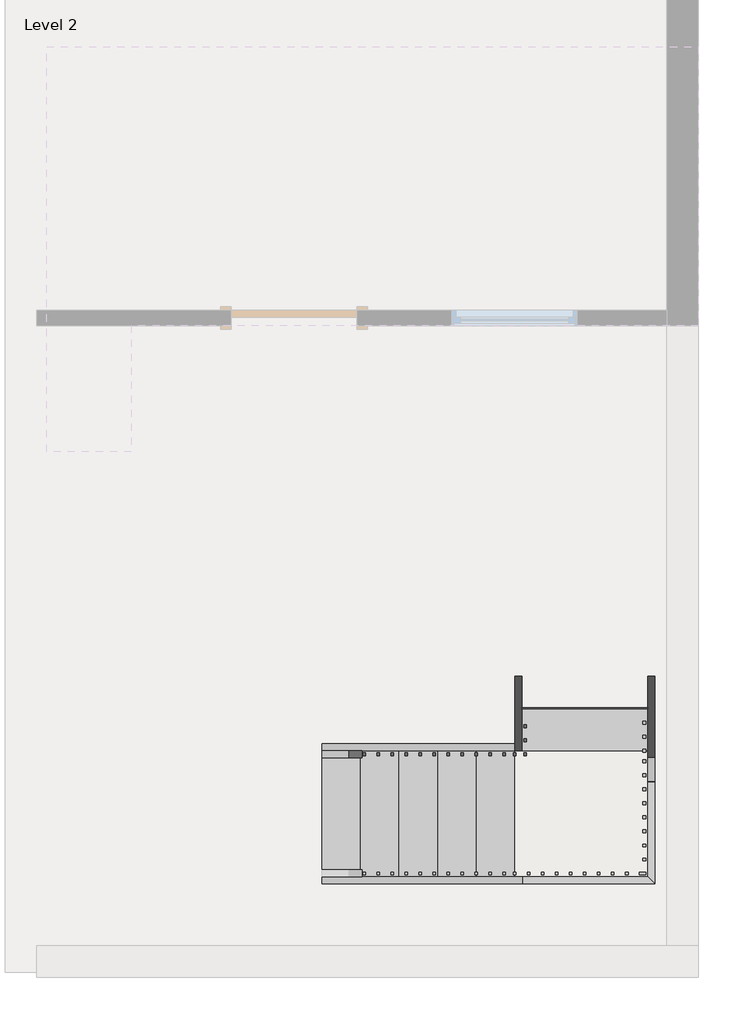
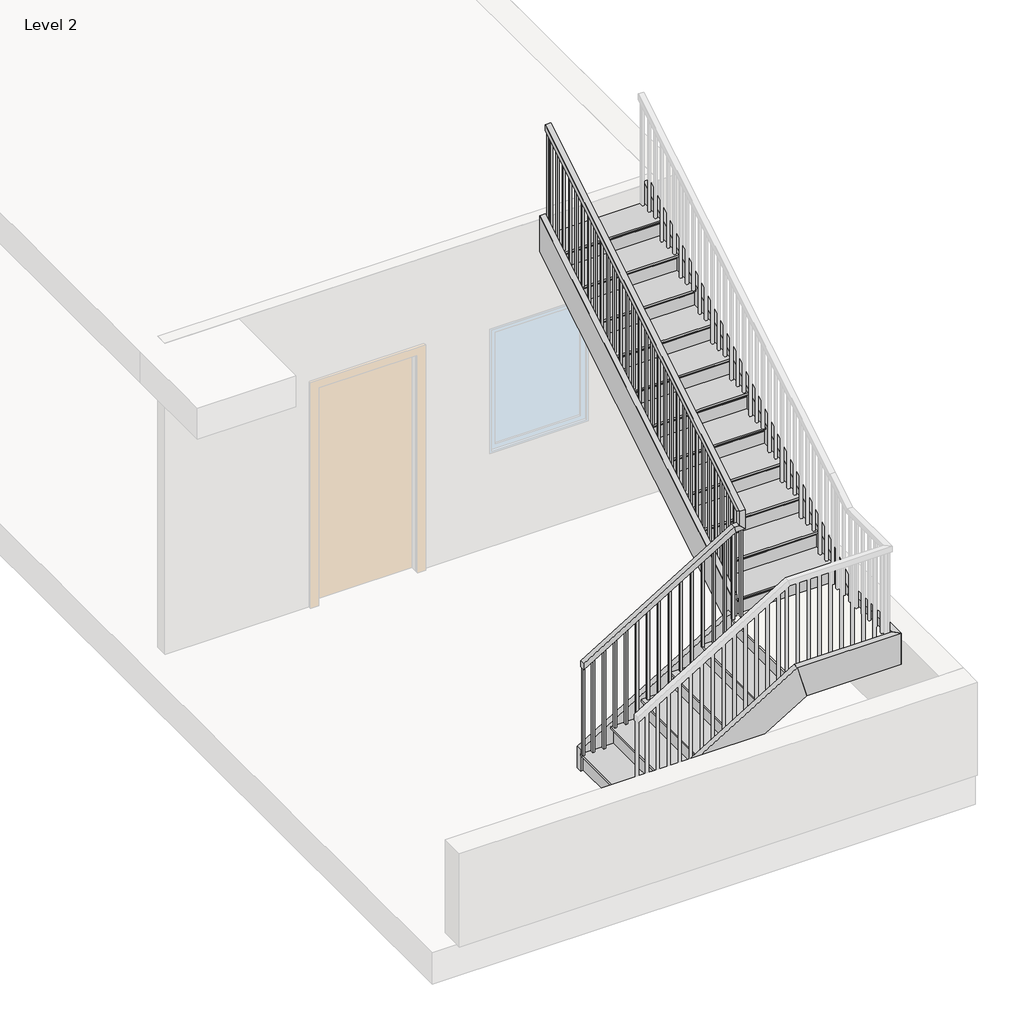
# One storey, part 2 of 2: 6 members, 2 stair flights, 1 railing, 1 slab.
"""IFC4 building model written with IfcOpenShell, lengths in millimetres."""

from ifc_helpers import new_model, si_unit, frame, origin, place, context, project, spatial, polyline, outline, extrude, faceted_brep, transform, mapped, element, save
from components import non_monolithic_landing_5acc3baf, stair_flight_09e20c57, stair_flight_b0062ef7

model = new_model("IFC4")

# Units and contexts
model_context = context("Model", 3, world=origin())
ifc_project = project(units=[si_unit("LENGTHUNIT", "METRE", prefix="MILLI")], contexts=[model_context])

# Site, building, storey
site = spatial("IfcSite", under=ifc_project)
building = spatial("IfcBuilding", under=site)
storey = spatial("IfcBuildingStorey", under=building, Name="Level 2", Elevation=3048.0)

# Members
placement = place(None, origin())
element("IfcMember", 1, ObjectType="Stringer - 2\" Width", at=placement, inside=storey, context=model_context, shape_type="SweptSolid", body=[
    extrude(outline(polyline([(3260.114512, -3351.0563134), (3048.0, -3351.0563134), (3048.0, -3112.9708017), (3750.3724171, -1954.0563134), (4106.7811786, -1954.0563134), (3260.114512, -3351.0563134)])), frame((0.0, -11795.059218, 0.0), z_axis=(0.0, 1.0, 0.0), x_axis=(0.0, 0.0, 1.0)), (0.0, 0.0, 1.0), 50.8),
])
element("IfcMember", 2, ObjectType="Stringer - 2\" Width", at=placement, inside=storey, context=model_context, shape_type="SweptSolid", body=[
    extrude(outline(polyline([(3260.114512, -3351.0563134), (3048.0, -3351.0563134), (3048.0, -3112.9708017), (3835.4, -1813.7608017), (4140.2, -1898.9152582), (3260.114512, -3351.0563134)])), frame((0.0, -12760.259218, 0.0), z_axis=(0.0, 1.0, 0.0), x_axis=(0.0, 0.0, 1.0)), (0.0, 0.0, 1.0), 50.8),
])
element("IfcMember", 3, ObjectType="Stringer - 2\" Width", at=placement, inside=storey, context=model_context, shape_type="SweptSolid", body=[
    extrude(outline(polyline([(-11795.059218, 3919.7057504), (-11795.059218, 4276.114512), (-8721.659218, 6138.7811786), (-8721.659218, 5782.3724171), (-11795.059218, 3919.7057504)])), frame((-1954.0563134, 0.0, 0.0), z_axis=(1.0, 0.0, 0.0), x_axis=(0.0, 1.0, 0.0)), (0.0, 0.0, 1.0), 50.8),
])
element("IfcMember", 4, ObjectType="Stringer - 2\" Width", at=placement, inside=storey, context=model_context, shape_type="SweptSolid", body=[
    extrude(outline(polyline([(-11934.1637062, 3835.4), (-12019.3181627, 4140.2), (-8721.659218, 6138.7811786), (-8721.659218, 5782.3724171), (-11934.1637062, 3835.4)])), frame((-988.8563134, 0.0, 0.0), z_axis=(1.0, 0.0, 0.0), x_axis=(0.0, 1.0, 0.0)), (0.0, 0.0, 1.0), 50.8),
])
element("IfcMember", 5, ObjectType="Stringer - 2\" Width", at=placement, inside=storey, context=model_context, shape_type="Brep", body=[
    faceted_brep([(-1898.9152582, -12709.459218, 4140.2), (-1898.9152582, -12760.259218, 4140.2), (-938.0563134, -12760.259218, 4140.2), (-988.8563134, -12709.459218, 4140.2), (-1813.7608017, -12709.459218, 3835.4), (-988.8563134, -12709.459218, 3835.4), (-1813.7608017, -12760.259218, 3835.4), (-938.0563134, -12760.259218, 3835.4)], [[[0, 1, 2, 3]], [[4, 0, 3, 5]], [[6, 4, 5, 7]], [[1, 6, 7, 2]], [[1, 0, 4, 6]], [[2, 7, 5, 3]]]),
])
element("IfcMember", 6, ObjectType="Stringer - 2\" Width", at=placement, inside=storey, context=model_context, shape_type="Brep", body=[
    faceted_brep([(-988.8563134, -12709.459218, 4140.2), (-938.0563134, -12760.259218, 4140.2), (-938.0563134, -12019.3181627, 4140.2), (-988.8563134, -12019.3181627, 4140.2), (-988.8563134, -12709.459218, 3835.4), (-988.8563134, -11934.1637062, 3835.4), (-938.0563134, -12760.259218, 3835.4), (-938.0563134, -11934.1637062, 3835.4)], [[[0, 1, 2, 3]], [[4, 0, 3, 5]], [[6, 4, 5, 7]], [[1, 6, 7, 2]], [[1, 0, 4, 6]], [[2, 7, 5, 3]]]),
])

# Railing
element("IfcRailing", 7, ObjectType="Handrail - Rectangular", at=placement, inside=storey, context=model_context, shape_type="SolidModel", body=[
    faceted_brep([(-3351.0563134, -11795.059218, 4131.7333333), (-3351.0563134, -11795.059218, 4072.3318731), (-3351.0563134, -11845.859218, 4072.3318731), (-3351.0563134, -11845.859218, 4131.7333333), (-1954.0563134, -11795.059218, 4978.4), (-1939.863904, -11795.059218, 4927.6), (-1939.863904, -11845.859218, 4927.6), (-1954.0563134, -11845.859218, 4978.4), (-1903.2563134, -11795.059218, 4978.4), (-1903.2563134, -11845.859218, 4978.4), (-1852.4563134, -11845.859218, 4927.6), (-1852.4563134, -11795.059218, 4927.6)], [[[0, 1, 2, 3]], [[1, 0, 4, 5]], [[2, 1, 5, 6]], [[3, 2, 6, 7]], [[0, 3, 7, 4]], [[8, 9, 10, 11]], [[5, 4, 8, 11]], [[6, 5, 11, 10]], [[7, 6, 10, 9]], [[4, 7, 9, 8]]]),
    faceted_brep([(-1903.2563134, -11795.059218, 4978.4), (-1852.4563134, -11795.059218, 4927.6), (-1852.4563134, -11845.859218, 4927.6), (-1903.2563134, -11845.859218, 4978.4), (-1903.2563134, -11795.059218, 5088.3318731), (-1903.2563134, -11845.859218, 5116.9454545), (-1852.4563134, -11845.859218, 5116.9454545), (-1852.4563134, -11795.059218, 5088.3318731)], [[[0, 1, 2, 3]], [[4, 5, 6, 7]], [[1, 0, 4, 7]], [[2, 1, 7, 6]], [[3, 2, 6, 5]], [[0, 3, 5, 4]]]),
    faceted_brep([(-1903.2563134, -11845.859218, 5116.9454545), (-1903.2563134, -11795.059218, 5088.3318731), (-1852.4563134, -11795.059218, 5088.3318731), (-1852.4563134, -11845.859218, 5116.9454545), (-1903.2563134, -8721.659218, 7010.4), (-1852.4563134, -8721.659218, 7010.4), (-1852.4563134, -8721.659218, 6950.9985397), (-1903.2563134, -8721.659218, 6950.9985397)], [[[0, 1, 2, 3]], [[4, 5, 6, 7]], [[1, 0, 4, 7]], [[2, 1, 7, 6]], [[3, 2, 6, 5]], [[0, 3, 5, 4]]]),
    extrude(outline(polyline([(-8762.934218, 6925.9833882), (-8762.934218, 5926.6666667), (-8781.984218, 5926.6666667), (-8781.984218, 6914.4379337), (-8762.934218, 6925.9833882)])), frame((-1887.3813134, 0.0, 0.0), z_axis=(1.0, 0.0, 0.0), x_axis=(0.0, 1.0, 0.0)), (0.0, 0.0, 1.0), 19.05),
    extrude(outline(polyline([(-8864.534218, 6864.4076307), (-8864.534218, 5926.6666667), (-8883.584218, 5926.6666667), (-8883.584218, 6852.8621761), (-8864.534218, 6864.4076307)])), frame((-1887.3813134, 0.0, 0.0), z_axis=(1.0, 0.0, 0.0), x_axis=(0.0, 1.0, 0.0)), (0.0, 0.0, 1.0), 19.05),
    extrude(outline(polyline([(-8966.134218, 6802.8318731), (-8966.134218, 5926.6666667), (-8985.184218, 5926.6666667), (-8985.184218, 6791.2864185), (-8966.134218, 6802.8318731)])), frame((-1887.3813134, 0.0, 0.0), z_axis=(1.0, 0.0, 0.0), x_axis=(0.0, 1.0, 0.0)), (0.0, 0.0, 1.0), 19.05),
    extrude(outline(polyline([(-9067.734218, 6741.2561155), (-9067.734218, 5757.3333333), (-9086.784218, 5757.3333333), (-9086.784218, 6729.710661), (-9067.734218, 6741.2561155)])), frame((-1887.3813134, 0.0, 0.0), z_axis=(1.0, 0.0, 0.0), x_axis=(0.0, 1.0, 0.0)), (0.0, 0.0, 1.0), 19.05),
    extrude(outline(polyline([(-9169.334218, 6679.6803579), (-9169.334218, 5757.3333333), (-9188.384218, 5757.3333333), (-9188.384218, 6668.1349034), (-9169.334218, 6679.6803579)])), frame((-1887.3813134, 0.0, 0.0), z_axis=(1.0, 0.0, 0.0), x_axis=(0.0, 1.0, 0.0)), (0.0, 0.0, 1.0), 19.05),
    extrude(outline(polyline([(-9270.934218, 6618.1046004), (-9270.934218, 5757.3333333), (-9289.984218, 5757.3333333), (-9289.984218, 6606.5591458), (-9270.934218, 6618.1046004)])), frame((-1887.3813134, 0.0, 0.0), z_axis=(1.0, 0.0, 0.0), x_axis=(0.0, 1.0, 0.0)), (0.0, 0.0, 1.0), 19.05),
    extrude(outline(polyline([(-9372.534218, 6556.5288428), (-9372.534218, 5588.0), (-9391.584218, 5588.0), (-9391.584218, 6544.9833882), (-9372.534218, 6556.5288428)])), frame((-1887.3813134, 0.0, 0.0), z_axis=(1.0, 0.0, 0.0), x_axis=(0.0, 1.0, 0.0)), (0.0, 0.0, 1.0), 19.05),
    extrude(outline(polyline([(-9474.134218, 6494.9530852), (-9474.134218, 5588.0), (-9493.184218, 5588.0), (-9493.184218, 6483.4076307), (-9474.134218, 6494.9530852)])), frame((-1887.3813134, 0.0, 0.0), z_axis=(1.0, 0.0, 0.0), x_axis=(0.0, 1.0, 0.0)), (0.0, 0.0, 1.0), 19.05),
    extrude(outline(polyline([(-9575.734218, 6433.3773276), (-9575.734218, 5418.6666667), (-9594.784218, 5418.6666667), (-9594.784218, 6421.8318731), (-9575.734218, 6433.3773276)])), frame((-1887.3813134, 0.0, 0.0), z_axis=(1.0, 0.0, 0.0), x_axis=(0.0, 1.0, 0.0)), (0.0, 0.0, 1.0), 19.05),
    extrude(outline(polyline([(-9677.334218, 6371.80157), (-9677.334218, 5418.6666667), (-9696.384218, 5418.6666667), (-9696.384218, 6360.2561155), (-9677.334218, 6371.80157)])), frame((-1887.3813134, 0.0, 0.0), z_axis=(1.0, 0.0, 0.0), x_axis=(0.0, 1.0, 0.0)), (0.0, 0.0, 1.0), 19.05),
    extrude(outline(polyline([(-9778.934218, 6310.2258125), (-9778.934218, 5418.6666667), (-9797.984218, 5418.6666667), (-9797.984218, 6298.6803579), (-9778.934218, 6310.2258125)])), frame((-1887.3813134, 0.0, 0.0), z_axis=(1.0, 0.0, 0.0), x_axis=(0.0, 1.0, 0.0)), (0.0, 0.0, 1.0), 19.05),
    extrude(outline(polyline([(-9880.534218, 6248.6500549), (-9880.534218, 5249.3333333), (-9899.584218, 5249.3333333), (-9899.584218, 6237.1046004), (-9880.534218, 6248.6500549)])), frame((-1887.3813134, 0.0, 0.0), z_axis=(1.0, 0.0, 0.0), x_axis=(0.0, 1.0, 0.0)), (0.0, 0.0, 1.0), 19.05),
    extrude(outline(polyline([(-9982.134218, 6187.0742973), (-9982.134218, 5249.3333333), (-10001.184218, 5249.3333333), (-10001.184218, 6175.5288428), (-9982.134218, 6187.0742973)])), frame((-1887.3813134, 0.0, 0.0), z_axis=(1.0, 0.0, 0.0), x_axis=(0.0, 1.0, 0.0)), (0.0, 0.0, 1.0), 19.05),
    extrude(outline(polyline([(-10083.734218, 6125.4985397), (-10083.734218, 5249.3333333), (-10102.784218, 5249.3333333), (-10102.784218, 6113.9530852), (-10083.734218, 6125.4985397)])), frame((-1887.3813134, 0.0, 0.0), z_axis=(1.0, 0.0, 0.0), x_axis=(0.0, 1.0, 0.0)), (0.0, 0.0, 1.0), 19.05),
    extrude(outline(polyline([(-10185.334218, 6063.9227822), (-10185.334218, 5080.0), (-10204.384218, 5080.0), (-10204.384218, 6052.3773276), (-10185.334218, 6063.9227822)])), frame((-1887.3813134, 0.0, 0.0), z_axis=(1.0, 0.0, 0.0), x_axis=(0.0, 1.0, 0.0)), (0.0, 0.0, 1.0), 19.05),
    extrude(outline(polyline([(-10286.934218, 6002.3470246), (-10286.934218, 5080.0), (-10305.984218, 5080.0), (-10305.984218, 5990.80157), (-10286.934218, 6002.3470246)])), frame((-1887.3813134, 0.0, 0.0), z_axis=(1.0, 0.0, 0.0), x_axis=(0.0, 1.0, 0.0)), (0.0, 0.0, 1.0), 19.05),
    extrude(outline(polyline([(-10388.534218, 5940.771267), (-10388.534218, 5080.0), (-10407.584218, 5080.0), (-10407.584218, 5929.2258125), (-10388.534218, 5940.771267)])), frame((-1887.3813134, 0.0, 0.0), z_axis=(1.0, 0.0, 0.0), x_axis=(0.0, 1.0, 0.0)), (0.0, 0.0, 1.0), 19.05),
    extrude(outline(polyline([(-10490.134218, 5879.1955094), (-10490.134218, 4910.6666667), (-10509.184218, 4910.6666667), (-10509.184218, 5867.6500549), (-10490.134218, 5879.1955094)])), frame((-1887.3813134, 0.0, 0.0), z_axis=(1.0, 0.0, 0.0), x_axis=(0.0, 1.0, 0.0)), (0.0, 0.0, 1.0), 19.05),
    extrude(outline(polyline([(-10591.734218, 5817.6197519), (-10591.734218, 4910.6666667), (-10610.784218, 4910.6666667), (-10610.784218, 5806.0742973), (-10591.734218, 5817.6197519)])), frame((-1887.3813134, 0.0, 0.0), z_axis=(1.0, 0.0, 0.0), x_axis=(0.0, 1.0, 0.0)), (0.0, 0.0, 1.0), 19.05),
    extrude(outline(polyline([(-10693.334218, 5756.0439943), (-10693.334218, 4741.3333333), (-10712.384218, 4741.3333333), (-10712.384218, 5744.4985397), (-10693.334218, 5756.0439943)])), frame((-1887.3813134, 0.0, 0.0), z_axis=(1.0, 0.0, 0.0), x_axis=(0.0, 1.0, 0.0)), (0.0, 0.0, 1.0), 19.05),
    extrude(outline(polyline([(-10794.934218, 5694.4682367), (-10794.934218, 4741.3333333), (-10813.984218, 4741.3333333), (-10813.984218, 5682.9227822), (-10794.934218, 5694.4682367)])), frame((-1887.3813134, 0.0, 0.0), z_axis=(1.0, 0.0, 0.0), x_axis=(0.0, 1.0, 0.0)), (0.0, 0.0, 1.0), 19.05),
    extrude(outline(polyline([(-10896.534218, 5632.8924791), (-10896.534218, 4741.3333333), (-10915.584218, 4741.3333333), (-10915.584218, 5621.3470246), (-10896.534218, 5632.8924791)])), frame((-1887.3813134, 0.0, 0.0), z_axis=(1.0, 0.0, 0.0), x_axis=(0.0, 1.0, 0.0)), (0.0, 0.0, 1.0), 19.05),
    extrude(outline(polyline([(-10998.134218, 5571.3167216), (-10998.134218, 4572.0), (-11017.184218, 4572.0), (-11017.184218, 5559.771267), (-10998.134218, 5571.3167216)])), frame((-1887.3813134, 0.0, 0.0), z_axis=(1.0, 0.0, 0.0), x_axis=(0.0, 1.0, 0.0)), (0.0, 0.0, 1.0), 19.05),
    extrude(outline(polyline([(-11099.734218, 5509.740964), (-11099.734218, 4572.0), (-11118.784218, 4572.0), (-11118.784218, 5498.1955094), (-11099.734218, 5509.740964)])), frame((-1887.3813134, 0.0, 0.0), z_axis=(1.0, 0.0, 0.0), x_axis=(0.0, 1.0, 0.0)), (0.0, 0.0, 1.0), 19.05),
    extrude(outline(polyline([(-11201.334218, 5448.1652064), (-11201.334218, 4572.0), (-11220.384218, 4572.0), (-11220.384218, 5436.6197519), (-11201.334218, 5448.1652064)])), frame((-1887.3813134, 0.0, 0.0), z_axis=(1.0, 0.0, 0.0), x_axis=(0.0, 1.0, 0.0)), (0.0, 0.0, 1.0), 19.05),
    extrude(outline(polyline([(-11302.934218, 5386.5894488), (-11302.934218, 4402.6666667), (-11321.984218, 4402.6666667), (-11321.984218, 5375.0439943), (-11302.934218, 5386.5894488)])), frame((-1887.3813134, 0.0, 0.0), z_axis=(1.0, 0.0, 0.0), x_axis=(0.0, 1.0, 0.0)), (0.0, 0.0, 1.0), 19.05),
    extrude(outline(polyline([(-11404.534218, 5325.0136913), (-11404.534218, 4402.6666667), (-11423.584218, 4402.6666667), (-11423.584218, 5313.4682367), (-11404.534218, 5325.0136913)])), frame((-1887.3813134, 0.0, 0.0), z_axis=(1.0, 0.0, 0.0), x_axis=(0.0, 1.0, 0.0)), (0.0, 0.0, 1.0), 19.05),
    extrude(outline(polyline([(-11506.134218, 5263.4379337), (-11506.134218, 4402.6666667), (-11525.184218, 4402.6666667), (-11525.184218, 5251.8924791), (-11506.134218, 5263.4379337)])), frame((-1887.3813134, 0.0, 0.0), z_axis=(1.0, 0.0, 0.0), x_axis=(0.0, 1.0, 0.0)), (0.0, 0.0, 1.0), 19.05),
    extrude(outline(polyline([(-11607.734218, 5201.8621761), (-11607.734218, 4233.3333333), (-11626.784218, 4233.3333333), (-11626.784218, 5190.3167216), (-11607.734218, 5201.8621761)])), frame((-1887.3813134, 0.0, 0.0), z_axis=(1.0, 0.0, 0.0), x_axis=(0.0, 1.0, 0.0)), (0.0, 0.0, 1.0), 19.05),
    extrude(outline(polyline([(-11709.334218, 5140.2864185), (-11709.334218, 4233.3333333), (-11728.384218, 4233.3333333), (-11728.384218, 5128.740964), (-11709.334218, 5140.2864185)])), frame((-1887.3813134, 0.0, 0.0), z_axis=(1.0, 0.0, 0.0), x_axis=(0.0, 1.0, 0.0)), (0.0, 0.0, 1.0), 19.05),
    extrude(outline(polyline([(4867.0439943, -2039.7813134), (3894.6666667, -2039.7813134), (3894.6666667, -2020.7313134), (4878.5894488, -2020.7313134), (4867.0439943, -2039.7813134)])), frame((0.0, -11829.984218, 0.0), z_axis=(0.0, 1.0, 0.0), x_axis=(0.0, 0.0, 1.0)), (0.0, 0.0, 1.0), 19.05),
    extrude(outline(polyline([(4805.4682367, -2141.3813134), (3894.6666667, -2141.3813134), (3894.6666667, -2122.3313134), (4817.0136913, -2122.3313134), (4805.4682367, -2141.3813134)])), frame((0.0, -11829.984218, 0.0), z_axis=(0.0, 1.0, 0.0), x_axis=(0.0, 0.0, 1.0)), (0.0, 0.0, 1.0), 19.05),
    extrude(outline(polyline([(4743.8924791, -2242.9813134), (3894.6666667, -2242.9813134), (3894.6666667, -2223.9313134), (4755.4379337, -2223.9313134), (4743.8924791, -2242.9813134)])), frame((0.0, -11829.984218, 0.0), z_axis=(0.0, 1.0, 0.0), x_axis=(0.0, 0.0, 1.0)), (0.0, 0.0, 1.0), 19.05),
    extrude(outline(polyline([(4682.3167216, -2344.5813134), (3725.3333333, -2344.5813134), (3725.3333333, -2325.5313134), (4693.8621761, -2325.5313134), (4682.3167216, -2344.5813134)])), frame((0.0, -11829.984218, 0.0), z_axis=(0.0, 1.0, 0.0), x_axis=(0.0, 0.0, 1.0)), (0.0, 0.0, 1.0), 19.05),
    extrude(outline(polyline([(4620.740964, -2446.1813134), (3725.3333333, -2446.1813134), (3725.3333333, -2427.1313134), (4632.2864185, -2427.1313134), (4620.740964, -2446.1813134)])), frame((0.0, -11829.984218, 0.0), z_axis=(0.0, 1.0, 0.0), x_axis=(0.0, 0.0, 1.0)), (0.0, 0.0, 1.0), 19.05),
    extrude(outline(polyline([(4559.1652064, -2547.7813134), (3556.0, -2547.7813134), (3556.0, -2528.7313134), (4570.710661, -2528.7313134), (4559.1652064, -2547.7813134)])), frame((0.0, -11829.984218, 0.0), z_axis=(0.0, 1.0, 0.0), x_axis=(0.0, 0.0, 1.0)), (0.0, 0.0, 1.0), 19.05),
    extrude(outline(polyline([(4497.5894488, -2649.3813134), (3556.0, -2649.3813134), (3556.0, -2630.3313134), (4509.1349034, -2630.3313134), (4497.5894488, -2649.3813134)])), frame((0.0, -11829.984218, 0.0), z_axis=(0.0, 1.0, 0.0), x_axis=(0.0, 0.0, 1.0)), (0.0, 0.0, 1.0), 19.05),
    extrude(outline(polyline([(4436.0136913, -2750.9813134), (3556.0, -2750.9813134), (3556.0, -2731.9313134), (4447.5591458, -2731.9313134), (4436.0136913, -2750.9813134)])), frame((0.0, -11829.984218, 0.0), z_axis=(0.0, 1.0, 0.0), x_axis=(0.0, 0.0, 1.0)), (0.0, 0.0, 1.0), 19.05),
    extrude(outline(polyline([(4374.4379337, -2852.5813134), (3386.6666667, -2852.5813134), (3386.6666667, -2833.5313134), (4385.9833882, -2833.5313134), (4374.4379337, -2852.5813134)])), frame((0.0, -11829.984218, 0.0), z_axis=(0.0, 1.0, 0.0), x_axis=(0.0, 0.0, 1.0)), (0.0, 0.0, 1.0), 19.05),
    extrude(outline(polyline([(4312.8621761, -2954.1813134), (3386.6666667, -2954.1813134), (3386.6666667, -2935.1313134), (4324.4076307, -2935.1313134), (4312.8621761, -2954.1813134)])), frame((0.0, -11829.984218, 0.0), z_axis=(0.0, 1.0, 0.0), x_axis=(0.0, 0.0, 1.0)), (0.0, 0.0, 1.0), 19.05),
    extrude(outline(polyline([(4251.2864185, -3055.7813134), (3386.6666667, -3055.7813134), (3386.6666667, -3036.7313134), (4262.8318731, -3036.7313134), (4251.2864185, -3055.7813134)])), frame((0.0, -11829.984218, 0.0), z_axis=(0.0, 1.0, 0.0), x_axis=(0.0, 0.0, 1.0)), (0.0, 0.0, 1.0), 19.05),
    extrude(outline(polyline([(4189.710661, -3157.3813134), (3217.3333333, -3157.3813134), (3217.3333333, -3138.3313134), (4201.2561155, -3138.3313134), (4189.710661, -3157.3813134)])), frame((0.0, -11829.984218, 0.0), z_axis=(0.0, 1.0, 0.0), x_axis=(0.0, 0.0, 1.0)), (0.0, 0.0, 1.0), 19.05),
    extrude(outline(polyline([(4128.1349034, -3258.9813134), (3217.3333333, -3258.9813134), (3217.3333333, -3239.9313134), (4139.6803579, -3239.9313134), (4128.1349034, -3258.9813134)])), frame((0.0, -11829.984218, 0.0), z_axis=(0.0, 1.0, 0.0), x_axis=(0.0, 0.0, 1.0)), (0.0, 0.0, 1.0), 19.05),
    extrude(outline(polyline([(-1887.3813134, -11810.934218), (-1868.3313134, -11810.934218), (-1868.3313134, -11829.984218), (-1887.3813134, -11829.984218), (-1887.3813134, -11810.934218)])), frame((0.0, 0.0, 4064.0), z_axis=(0.0, 0.0, 1.0), x_axis=(1.0, 0.0, 0.0)), (0.0, 0.0, 1.0), 863.6),
    extrude(outline(polyline([(4913.2258125, -1963.5813134), (4064.0, -1963.5813134), (4064.0, -1944.5313134), (4924.771267, -1944.5313134), (4913.2258125, -1963.5813134)])), frame((0.0, -11829.984218, 0.0), z_axis=(0.0, 1.0, 0.0), x_axis=(0.0, 0.0, 1.0)), (0.0, 0.0, 1.0), 19.05),
    extrude(outline(polyline([(-8721.659218, 6950.9985397), (-8721.659218, 5926.6666667), (-8740.709218, 5926.6666667), (-8740.709218, 6939.4530852), (-8721.659218, 6950.9985397)])), frame((-1887.3813134, 0.0, 0.0), z_axis=(1.0, 0.0, 0.0), x_axis=(0.0, 1.0, 0.0)), (0.0, 0.0, 1.0), 19.05),
    extrude(outline(polyline([(4072.3318731, -3351.0563134), (3217.3333333, -3351.0563134), (3217.3333333, -3332.0063134), (4083.8773276, -3332.0063134), (4072.3318731, -3351.0563134)])), frame((0.0, -11829.984218, 0.0), z_axis=(0.0, 1.0, 0.0), x_axis=(0.0, 0.0, 1.0)), (0.0, 0.0, 1.0), 19.05),
])

# Slab
non_monolithic_landing_shape = non_monolithic_landing_5acc3baf(model_context)
element("IfcSlab", 8, ObjectType="Non-Monolithic Landing", at=placement, inside=storey, context=model_context, shape_type="MappedRepresentation", body=[
    mapped(non_monolithic_landing_shape, transform((0.0, 0.0, 0.0), x_axis=(1.0, 0.0, 0.0), y_axis=(0.0, 1.0, 0.0), z_axis=(0.0, 0.0, 1.0))),
])

# Stair flights
stair_flight_shape = stair_flight_09e20c57(model_context)
element("IfcStairFlight", 9, ObjectType="2\" Tread 1\" Nosing 1/4\" Riser", at=placement, inside=storey, context=model_context, shape_type="MappedRepresentation", body=[
    mapped(stair_flight_shape, transform((0.0, 0.0, 0.0), x_axis=(1.0, 0.0, 0.0), y_axis=(0.0, 1.0, 0.0), z_axis=(0.0, 0.0, 1.0))),
])
stair_flight_2_shape = stair_flight_b0062ef7(model_context)
element("IfcStairFlight", 10, ObjectType="2\" Tread 1\" Nosing 1/4\" Riser", at=placement, inside=storey, context=model_context, shape_type="MappedRepresentation", body=[
    mapped(stair_flight_2_shape, transform((0.0, 0.0, 0.0), x_axis=(1.0, 0.0, 0.0), y_axis=(0.0, 1.0, 0.0), z_axis=(0.0, 0.0, 1.0))),
])

save(model, "model.ifc")

# Revit data of these elements
# Type "Handrail - Rectangular"
#   Assembly Code = "C2010400"
#   built-in parameter 1008612 = 0.0416667 (stored number, unit not read)
#   built-in parameter 1008611 = 0.0416667 (stored number, unit not read)
#   built-in parameter 1008609 = 0.333333 (stored number, unit not read)
#   built-in parameter 1008604 = 0.166667 (stored number, unit not read)
#   built-in parameter 1008603 = 0.166667 (stored number, unit not read)
#   Railing Height = 3' - 0"
#   built-in parameter 1008630 = 2
#   built-in parameter 1008610 = 2
#   built-in parameter 1008618 = Baluster - Square : 3/4"
# Elements 1, 2, 3, 4, 5, 6 (IfcMember, "Stringer - 2\" Width")
#   Phase Created = New Construction
# Element 7 (IfcRailing, "Handrail - Rectangular")
#   Phase Created = New Construction
# Element 8 (IfcSlab, "Non-Monolithic Landing")
#   Phase Created = New Construction
# Elements 9, 10 (IfcStairFlight, "2\" Tread 1\" Nosing 1/4\" Riser")
#   Phase Created = New Construction
